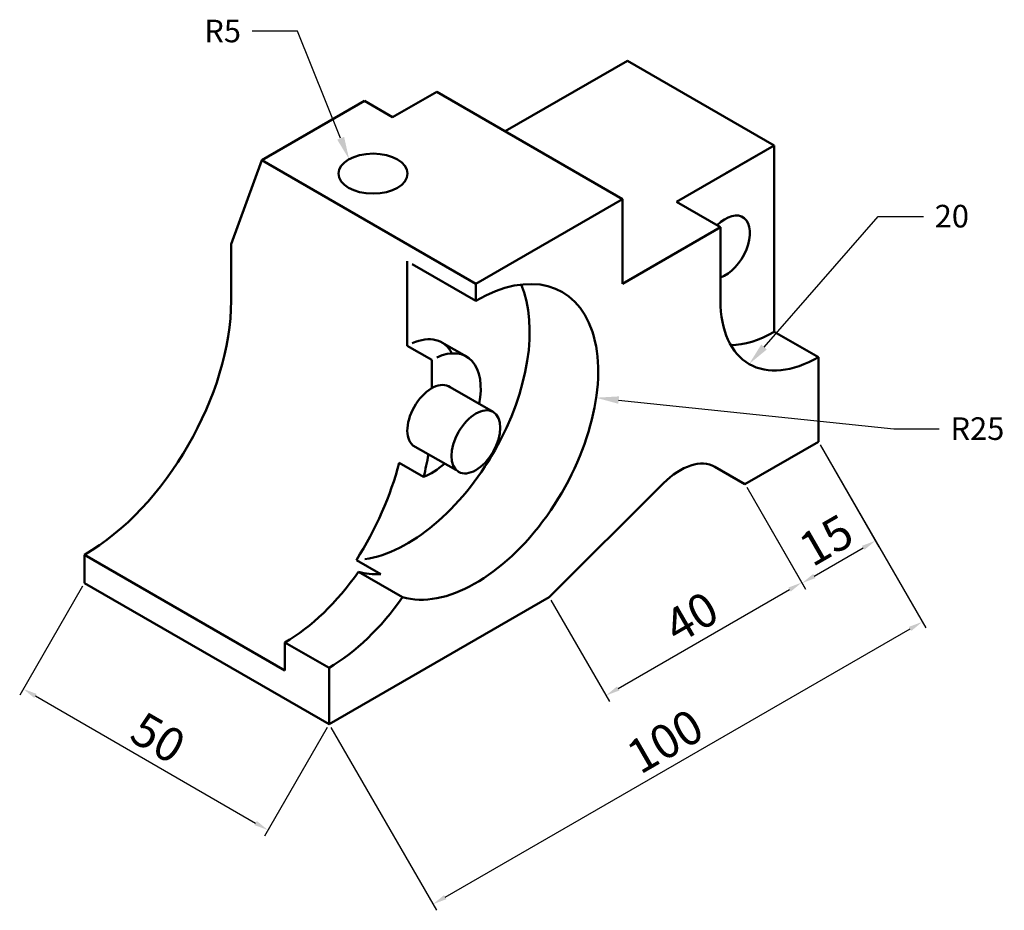
# Model space of a CAD drawing. Units: millimetres. Extents: x 2329 to 2503, y 1163 to 1320.
import ezdxf
from ezdxf import colors
from ezdxf.entities.mleader import LeaderData, LeaderLine
from ezdxf.math import Vec2, Vec3

# ---------------------------------------------------------------- set-up
doc = ezdxf.new("R2010")
doc.units = ezdxf.units.MM
doc.layers.add('M-DIMS', color=2, linetype='Continuous', lineweight=25)
doc.layers.add('M-OUTL', color=7, linetype='Continuous', lineweight=50)
doc.styles.get("Standard").update_dxf_attribs({"font": 'arial.ttf'})
doc.dimstyles.new('ISO-25', dxfattribs={"dimtxt": 6, "dimasz": 2.5, "dimexe": 1.25, "dimexo": 0.625, "dimtad": 1, "dimtxsty": 'Standard', "dimcen": 2.5, "dimadec": 0, "dimazin": 0, "dimtfac": 1, "dimtmove": 0, "dimatfit": 3, "dimfxl": 1, "dimarcsym": 0})

# ---------------------------------------------------------------- blocks, each defined once
blk = doc.blocks.new('*D1')
at = {"layer": 'Defpoints', "color": 0, "transparency": 16777216}
for p in [(2456.95, 1237.97), (2467, 1220.56), (2422.31, 1217.97)]:
    blk.add_point(p, dxfattribs=at)
at = {"layer": 'M-DIMS', "color": 0, "lineweight": -2, "transparency": 16777216}
for p, q in [((2457.26, 1237.42), (2467.62, 1219.48)), ((2434.52, 1201.81), (2464.83, 1219.31)), ((2422.62, 1217.42), (2432.98, 1199.48))]:
    blk.add_line(p, q, dxfattribs=at)
at = {"layer": 'M-DIMS', "color": 0, "transparency": 16777216}
for points in [[(2464.63, 1219.67), (2465.04, 1218.95), (2467, 1220.56)], [(2434.31, 1202.17), (2434.73, 1201.45), (2432.36, 1200.56)]]:
    blk.add_solid(points, dxfattribs=at)
at = {"layer": 'M-DIMS', "color": 0, "transparency": 16777216, "insert": (2447.83, 1213.75), "char_height": 6, "attachment_point": 5, "rotation": 30}
blk.add_mtext('40', dxfattribs=at)
blk = doc.blocks.new('*D2')
at = {"layer": 'Defpoints', "color": 0, "transparency": 16777216}
for p in [(2469.94, 1245.47), (2456.95, 1237.97), (2480.05, 1227.96)]:
    blk.add_point(p, dxfattribs=at)
at = {"layer": 'M-DIMS', "color": 0, "lineweight": -2, "transparency": 16777216}
for p, q in [((2470.25, 1244.92), (2480.67, 1226.88)), ((2457.26, 1237.42), (2467.68, 1219.38)), ((2469.22, 1221.71), (2477.88, 1226.71))]:
    blk.add_line(p, q, dxfattribs=at)
at = {"layer": 'M-DIMS', "color": 0, "transparency": 16777216}
for points in [[(2477.67, 1227.07), (2478.09, 1226.35), (2480.05, 1227.96)], [(2469.01, 1222.07), (2469.43, 1221.35), (2467.06, 1220.46)]]:
    blk.add_solid(points, dxfattribs=at)
at = {"layer": 'M-DIMS', "color": 0, "transparency": 16777216, "insert": (2471.71, 1227.4), "char_height": 6, "attachment_point": 5, "rotation": 30}
blk.add_mtext('15', dxfattribs=at)
blk = doc.blocks.new('*D3')
at = {"layer": 'Defpoints', "color": 0, "transparency": 16777216}
for p in [(2469.94, 1245.47), (2488.34, 1213.6), (2383.34, 1195.47)]:
    blk.add_point(p, dxfattribs=at)
at = {"layer": 'M-DIMS', "color": 0, "lineweight": -2, "transparency": 16777216}
for p, q in [((2470.25, 1244.92), (2488.96, 1212.52)), ((2403.9, 1164.85), (2486.17, 1212.35)), ((2383.65, 1194.92), (2402.36, 1162.52))]:
    blk.add_line(p, q, dxfattribs=at)
at = {"layer": 'M-DIMS', "color": 0, "transparency": 16777216}
for points in [[(2485.96, 1212.71), (2486.38, 1211.99), (2488.34, 1213.6)], [(2403.69, 1165.21), (2404.11, 1164.49), (2401.73, 1163.6)]]:
    blk.add_solid(points, dxfattribs=at)
at = {"layer": 'M-DIMS', "color": 0, "transparency": 16777216, "insert": (2443.19, 1191.8), "char_height": 6, "attachment_point": 5, "rotation": 30}
blk.add_mtext('100', dxfattribs=at)
blk = doc.blocks.new('*D4')
at = {"layer": 'Defpoints', "color": 0, "transparency": 16777216}
for p in [(2340.03, 1220.47), (2383.34, 1195.47), (2372.52, 1176.73)]:
    blk.add_point(p, dxfattribs=at)
at = {"layer": 'M-DIMS', "color": 0, "lineweight": -2, "transparency": 16777216}
for p, q in [((2339.72, 1219.92), (2328.59, 1200.64)), ((2331.38, 1200.48), (2370.35, 1177.98)), ((2383.02, 1194.92), (2371.89, 1175.64))]:
    blk.add_line(p, q, dxfattribs=at)
at = {"layer": 'M-DIMS', "color": 0, "transparency": 16777216}
for points in [[(2331.59, 1200.84), (2331.17, 1200.11), (2329.22, 1201.73)], [(2370.56, 1178.34), (2370.14, 1177.61), (2372.52, 1176.73)]]:
    blk.add_solid(points, dxfattribs=at)
at = {"layer": 'M-DIMS', "color": 0, "transparency": 16777216, "insert": (2352.71, 1192.42), "char_height": 6, "attachment_point": 5, "rotation": 330}
blk.add_mtext('50', dxfattribs=at)

msp = doc.modelspace()

# ---------------------------------------------------------------- linework, layer by layer
at = {"layer": 'M-OUTL'}
for p, q in [((2436.164, 1312.966), (2414.513, 1300.466)), ((2462.144, 1297.966), (2436.164, 1312.966)), ((2402.389, 1307.466), (2394.594, 1302.966)), ((2435.298, 1288.466), (2402.389, 1307.466)), ((2371.429, 1295.34), (2389.616, 1305.84)), ((2394.594, 1302.966), (2389.616, 1305.84)), ((2371.429, 1295.34), (2379.224, 1299.84)), ((2462.144, 1297.966), (2444.824, 1287.966)), ((2462.144, 1297.966), (2453.484, 1292.966)), ((2462.144, 1264.966), (2462.144, 1297.966)), ((2366.016, 1280.466), (2371.429, 1295.34)), ((2371.429, 1295.34), (2409.317, 1273.466)), ((2409.317, 1273.466), (2435.298, 1288.466)), ((2435.298, 1273.466), (2435.298, 1288.466)), ((2444.824, 1287.966), (2452.618, 1283.466)), ((2452.618, 1283.466), (2435.298, 1273.466)), ((2452.618, 1283.466), (2452.618, 1270.466)), ((2366.016, 1270.466), (2366.016, 1280.466)), ((2397.192, 1262.466), (2397.192, 1277.466)), ((2409.317, 1270.466), (2398.077, 1276.956)), ((2409.317, 1273.466), (2409.317, 1270.466)), ((2409.317, 1273.466), (2409.317, 1271.466)), ((2469.939, 1260.466), (2462.144, 1264.966)), ((2401.523, 1259.966), (2397.192, 1262.466)), ((2407.646, 1260.573), (2403.316, 1263.073)), ((2401.523, 1254.966), (2401.523, 1259.966)), ((2469.939, 1245.466), (2469.939, 1260.466)), ((2404.781, 1255.14), (2412.379, 1250.769)), ((2405.805, 1240.514), (2398.185, 1244.853)), ((2456.948, 1237.966), (2469.939, 1245.466)), ((2400.079, 1239.273), (2395.749, 1241.773)), ((2451.606, 1241.051), (2456.948, 1237.966)), ((2422.307, 1217.966), (2442.52, 1238.131)), ((2340.035, 1220.466), (2340.035, 1225.466)), ((2340.035, 1220.466), (2340.035, 1225.466)), ((2340.035, 1225.466), (2375.542, 1204.966)), ((2388.171, 1224.531), (2392.501, 1222.031)), ((2388.532, 1222.466), (2396.326, 1217.966)), ((2383.336, 1195.466), (2340.035, 1220.466)), ((2383.336, 1195.466), (2422.307, 1217.966)), ((2375.542, 1209.966), (2375.542, 1204.966)), ((2383.336, 1205.466), (2375.542, 1209.966)), ((2383.336, 1205.466), (2383.336, 1195.466))]:
    msp.add_line(p, q, dxfattribs=at)
for centre, major_axis in [((2391.13, 1292.966), (-6.124, 0)), ((2409.317, 1245.466), (-3.062, -5.303))]:
    msp.add_ellipse(centre, major_axis=major_axis, ratio=0.5773503, dxfattribs=at)
for centre, major_axis, start_param, end_param in [((2453.484, 1279.966), (-3.062, -5.303), 6.8672255, 10.5574253), ((2409.317, 1245.466), (-15.309, -26.517), 6.4250824, 10.2101761), ((2397.193, 1252.466), (-15.309, -26.517), 6.7147799, 9.0176433), ((2340.035, 1255.466), (18.371, 31.82), 3.9269912, 5.4977868), ((2469.939, 1280.466), (-12.247, -21.213), 5.4977871, 7.0685835), ((2397.193, 1252.466), (-6.124, -10.607), 9.0634108, 10.1079128), ((2462.144, 1284.966), (-12.247, -21.213), 6.6070134, 7.0685835), ((2401.523, 1249.966), (-6.124, -10.607), 8.3771639, 10.1079128), ((2401.523, 1249.966), (-3.062, -5.303), 3.0752472, 6.1886112), ((2375.542, 1234.966), (-18.371, -31.82), 2.0212981, 2.1417562), ((2371.212, 1237.466), (-18.371, -31.82), 1.4966436, 2.0212981), ((2401.523, 1249.966), (6.124, 10.607), 3.7595424, 4.1887902), ((2445.482, 1230.444), (-6.124, -10.607), 3.1415966, 4.2760646), ((2375.542, 1234.966), (-15.309, -26.517), 7.0685835, 7.7120846), ((2401.523, 1249.966), (15.309, 26.517), 3.2834914, 3.4972152), ((2383.336, 1230.466), (-15.309, -26.517), 7.0685835, 7.7120846)]:
    msp.add_ellipse(centre, major_axis=major_axis, ratio=0.5773503, start_param=start_param, end_param=end_param, dxfattribs=at)

# ---------------------------------------------------------------- dimensions: what is measured, and where the dimension line sits
at = {"layer": 'M-DIMS'}
for p1, p2, distance, picture, middle in [((2383.336, 1195.466), (2469.939, 1245.466), -36.794, '*D3', (2443.19, 1191.796)), ((2456.948, 1237.966), (2469.939, 1245.466), -20.214, '*D2', (2471.706, 1227.404)), ((2422.307, 1217.966), (2456.948, 1237.966), -20.101, '*D1', (2447.834, 1213.752)), ((2340.035, 1220.466), (2383.336, 1195.466), -21.64, '*D4', (2352.71, 1192.42))]:
    dim = msp.add_aligned_dim(p1=p1, p2=p2, distance=distance, dimstyle='ISO-25', override={"dimclrd": 0, "dimclre": 0, "dimclrt": 0}, dxfattribs=at)
    dim.commit()
    dim.dimension.update_dxf_attribs({"geometry": picture, "text_midpoint": middle})

# ---------------------------------------------------------------- leaders
ml = msp.add_multileader_mtext('Standard', dxfattribs=at)
ml.set_content('R5', color=256)
ml.set_leader_properties()
ml.build(insert=Vec2(0, 0))
ctx = ml.context
ctx.base_point, ctx.plane_origin = Vec3(2359.27, 1318.191), Vec3(2386.892, 1295.518)
ctx.text_align_type = 2
notes = []
notes.append((ctx, [(0, (1, 1, 0), (2377.75, 1318.191), (-1, 0), 8, [(0, [(2386.892, 1295.518)], 0, [])])]))
ctx.mtext.insert, ctx.mtext.alignment, ctx.mtext.flow_direction = Vec3(2367.75, 1320.225), 3, 5
ml = msp.add_multileader_mtext('Standard', dxfattribs=at)
ml.set_content('20', color=256)
ml.set_leader_properties()
ml.build(insert=Vec2(0, 0))
ctx = ml.context
ctx.base_point, ctx.plane_origin = Vec3(2488.538, 1285.402), Vec3(2457.691, 1259.253)
notes.append((ctx, [(0, (1, 1, 0), (2480.538, 1285.402), (1, 0), 8, [(0, [(2457.691, 1259.253)], 0, [])])]))
ctx.mtext.insert, ctx.mtext.flow_direction = Vec3(2490.538, 1287.436), 5
ml = msp.add_multileader_mtext('Standard', dxfattribs=at)
ml.set_content('R25', color=256)
ml.set_leader_properties()
ml.build(insert=Vec2(0, 0))
ctx = ml.context
ctx.base_point, ctx.plane_origin = Vec3(2491.327, 1247.78), Vec3(2430.617, 1253.284)
notes.append((ctx, [(0, (1, 1, 0), (2483.327, 1247.78), (1, 0), 8, [(0, [(2430.617, 1253.284)], 0, [])])]))
ctx.mtext.insert, ctx.mtext.flow_direction = Vec3(2493.327, 1249.814), 5
for ctx, leaders in notes:
    for number, flags, end, landing, length, lines in leaders:
        leader = LeaderData()
        leader.index, (leader.has_last_leader_line, leader.has_dogleg_vector, leader.attachment_direction) = number, flags
        leader.last_leader_point, leader.dogleg_vector, leader.dogleg_length = Vec3(end), Vec3(landing), length
        for number, points, colour, breaks in lines:
            line = LeaderLine()
            line.index, line.vertices, line.color, line.breaks = number, Vec3.list(points), colors.encode_raw_color(colour), breaks
            leader.lines.append(line)
        ctx.leaders.append(leader)

doc.saveas('drawing.dxf')
